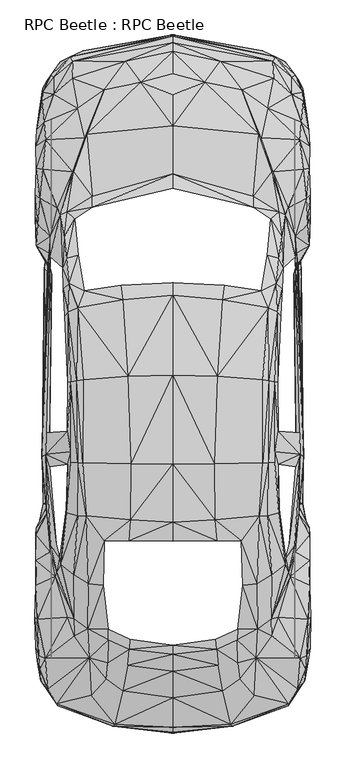
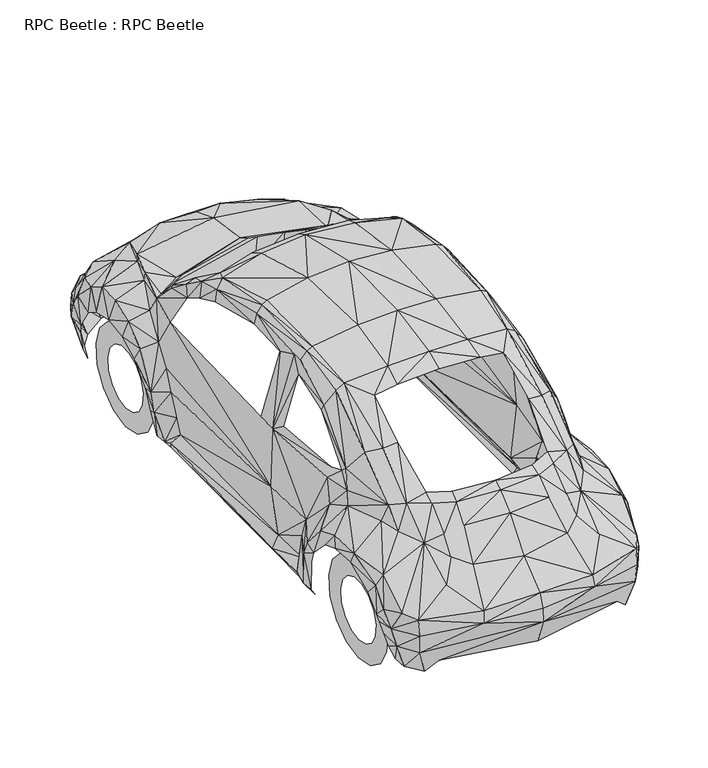
"""IFC4 building model written with IfcOpenShell, lengths in millimetres: proxy geometry, RPC Beetle : RPC Beetle."""

from ifc_helpers import new_model, si_unit, origin, place, context, project, spatial, triangles, source, transform, mapped, element, save


def rpc_beetle_rpc_beetle_31f8b51e(model_context):
    return source(origin(), model_context, "Body", "Tessellation", [
        triangles([(0.0, -748.5640469, 521.3894322), (0.0, -720.14536, 603.624202), (0.0, -696.6746996, 283.1362969), (0.0, -552.698168, 738.4051466), (0.0, -753.249444, 438.4540512), (0.0, -253.6666567, 1039.7136446), (0.0, -401.1024794, 921.3971746), (0.0, -304.8115909, 1012.258271), (0.0, 339.3169338, 1395.7139351), (0.0, 448.6129515, 1442.1297066), (0.0, 778.077507, 1504.0467121), (0.0, 1285.0167675, 1509.4764679), (0.0, 1741.0736687, 1402.3260315), (0.0, 2430.9612099, 967.1999022), (0.0, 3130.000518, 632.0428888), (0.0, 3001.4374352, 771.5092306), (0.0, 2704.2451103, 928.7536297), (0.0, 3164.1993027, 220.1684652), (0.0, 2883.1647125, 858.7358831), (0.0, 3222.5256844, 395.8040746), (0.0, 3178.9998528, 555.7633879), (0.0, 3213.9430687, 530.2784972), (-338.1784132, -715.5037828, 523.0096095), (-331.0409128, -702.1482754, 593.4652654), (-244.7338081, -218.0228295, 1034.0649342), (-248.9812959, -275.9549947, 1002.9312967), (-257.7389917, -368.17353, 911.8513184), (-249.0688632, 342.8199903, 1381.001025), (-285.238149, -511.5370176, 760.4306917), (-240.1360146, 460.0855433, 1426.5848705), (-236.4577871, 780.8799522, 1493.4060825), (-652.4921494, -590.2249108, 370.4943186), (-540.0870918, -593.333878, 283.4428189), (-181.240518, 2954.2772324, 806.3210592), (-253.1849819, 1278.5798058, 1496.1647804), (-379.8650402, -444.3655, 798.2639929), (-370.9321916, -353.3292326, 889.1688366), (-367.9983953, -222.2265337, 1003.4567734), (-368.3924847, -160.7037264, 1036.6922447), (-390.1553641, 342.863774, 1359.0192272), (-282.5670547, 1713.2680984, 1399.3047043), (-397.3366482, 87.4893818, 1215.3492176), (-463.1069432, -537.7663033, 704.8193333), (-271.4885704, 3072.331073, 662.6948696), (-475.7618394, -323.0714138, 849.8468182), (-463.7199872, 3085.9055351, 214.2570346), (-482.2425121, 95.7654028, 1203.3950054), (-485.0449937, -159.3024857, 1005.0769506), (-568.7247697, 3071.499147, 546.7429356), (-493.539933, 483.2496454, 1391.2913853), (-583.2625451, 3099.3922119, 522.0462599), (-510.267146, 3132.2774139, 369.399618), (-391.8631087, 2911.6272194, 782.7628315), (-656.3455479, -597.8441042, 480.0968946), (-660.2426937, -584.8389387, 576.2563957), (-562.2878443, -200.0695649, 879.7105476), (-560.0546594, -101.457906, 987.167506), (-512.4565836, 786.1783207, 1448.435281), (-541.7948364, 484.7822554, 1359.8511532), (-563.9956252, 148.5743069, 1172.305188), (-608.4846974, -561.2369273, 218.4607206), (-511.2742793, 1258.5246346, 1456.1858253), (-542.4078804, 784.6895308, 1430.657151), (-458.8594554, 2304.0621243, 949.0276829), (-601.0406751, -92.7440029, 893.1973698), (-503.7426533, 1765.2887604, 1320.9670441), (-546.0423243, 1253.0073841, 1441.5166626), (-603.011158, 501.1591264, 1278.5798058), (-580.1535416, 788.8932713, 1378.7239838), (-607.2148258, 519.8568223, 1235.1416142), (-601.2595934, 965.2732029, 1337.0374294), (-712.4823103, -503.0858256, 590.4876492), (-542.6706187, 1670.0487888, 1361.1648811), (-490.6061368, 2657.8732315, 893.5038918), (-599.6394161, 778.077507, 1307.3050873), (-598.0630589, 1243.7242298, 1343.7809132), (-639.5745512, 208.1266494, 1062.483621), (-680.4291796, -470.2006963, 218.6796571), (-538.4669146, 1966.7157097, 1180.581209), (-580.9855402, 1248.2344196, 1401.7567348), (-644.5226503, 243.2887836, 1028.2848364), (-502.3414307, 2635.8036484, 866.0047709), (-660.7243504, 162.2363182, 955.24569), (-690.2378105, -396.5922532, 226.8243271), (-559.1350934, 2175.0175301, 1011.1635704), (-670.1826393, 140.8675371, 872.7043619), (-662.475915, 324.2974654, 1009.4558258), (-615.0967575, 1623.4578827, 1262.1154037), (-594.6475333, 1646.0964718, 1321.2735661), (-589.4367322, 1809.6026253, 1269.4280388), (-728.8154703, -481.9797738, 373.2091965), (-751.5854467, -454.4368329, 476.550018), (-694.047389, 315.3208331, 957.7854332), (-726.5822491, -327.3188653, 735.5588814), (-622.9348692, 1777.2429726, 1192.7981958), (-564.6524529, 2445.7178673, 934.1396381), (-731.7930502, -393.8773753, 324.1223308), (-571.0017746, 2444.2728973, 884.1769901), (-698.6452188, 279.8521769, 807.6347145), (-604.2809933, 1949.769651, 1170.4660561), (-587.4224293, 3013.0852707, 200.1133485), (-690.9384218, 574.2421291, 283.6179717), (-750.2280441, -381.0035608, 396.9863425), (-627.532699, 1896.2601265, 1124.7070759), (-602.4856813, 2215.5656364, 949.1590702), (-619.4318127, 2072.8151928, 1075.2699045), (-710.4680437, 549.6329844, 448.6129515), (-764.7219995, -360.335382, 467.5296021), (-699.5209648, 762.6201656, 1015.4986256), (-763.3207769, -313.2189992, 670.9270706), (-757.8472012, -390.9435428, 564.6524529), (-717.4742294, 496.2986309, 583.5690671), (-722.7288506, 461.224064, 180.9777796), (-717.6493641, 554.4497326, 179.883079), (-771.4654106, -341.8128571, 511.011541), (-573.9356071, 2975.4709969, 682.6185808), (-730.7859169, 375.8802907, 185.1814838), (-541.1818288, 2805.3964943, 782.9380388), (-639.7496859, 2198.4444431, 944.2547911), (-738.9305506, 551.5596837, 222.4016865), (-781.5805635, -268.7736925, 609.2290924), (-772.2974092, -106.0556994, 755.9205019), (-721.7217173, 957.7416132, 967.0247675), (-703.3305433, 810.1306377, 292.3318839), (-724.8306845, 835.0462681, 964.3537096), (-757.7596338, 370.5381022, 225.46687), (-785.3463947, -89.9415395, 695.4924316), (-779.6538643, 80.9211054, 675.5686478), (-779.3911623, 89.5036484, 754.6506666), (-760.3869444, 444.1027617, 223.1460814), (-778.077507, 192.1000659, 630.9044409), (-658.6225164, 2237.1534176, 849.7592508), (-770.939934, 345.4910846, 426.1932807), (-774.1802885, 315.1456985, 501.684603), (-781.1864742, 232.2541011, 695.886521), (-719.225794, 810.0868904, 185.8383114), (-689.8874685, 1858.8647346, 293.9082775), (-696.6746996, 1958.8776707, 956.4279579), (-779.7414316, 377.369117, 532.3803311), (-778.1212543, 416.9976937, 439.7239228), (-745.498827, 819.5889267, 613.6517149), (-677.7143017, 2884.8288551, 670.6205486), (-697.5504456, 2077.4130226, 756.8838879), (-639.6182985, 3069.1783585, 391.6879377), (-713.0077869, 1918.2419243, 536.7153863), (-718.1748407, 1909.878336, 192.97583), (-705.1696753, 1981.9541691, 648.2884089), (-730.7859169, 1891.093, 233.3488017), (-673.9922905, 2907.8614609, 198.6683241), (-726.8887711, 2038.9229301, 189.9544301), (-721.6341499, 1973.3715534, 189.9544301), (-678.1959583, 2982.5647499, 540.5250011), (-699.6085321, 2815.6868546, 206.1999501), (-696.3681776, 2991.5851295, 517.4046827), (-723.6484165, 2624.6813622, 787.579616), (-699.0830555, 1882.4667824, 390.3742825), (-764.8971342, 2042.1632847, 362.5686032), (-741.7768158, 2457.6720795, 808.6856678), (-716.1605742, 2965.1367439, 449.5325174), (-766.4297441, 2001.1335217, 376.580902), (-731.5740955, 2724.4316689, 727.6331297), (-771.1588886, 2084.5942703, 482.2425121), (-759.1171091, 2291.4073734, 780.0917736), (-769.0132347, 2143.3146687, 699.0393082), (-777.5520304, 2022.8525448, 494.8098046), (-742.4774271, 2846.864312, 601.8726374), (-782.1060402, 2185.6581596, 616.4542328), (-739.5435946, 2918.4145958, 427.3755486), (-741.1200245, 2896.5202927, 519.8130386), (-750.4031788, 2804.433181, 398.0810795), (-782.2373549, 2313.1701439, 680.7357016), (-778.077507, 2462.7953133, 693.5219124), (-759.9052877, 2786.6113037, 455.2250115), (-774.1802885, 2682.8324638, 602.6608523), (-780.3544756, 2589.4317696, 666.3293135), (-742.6088144, 809.1235044, 220.3874199), (0.0, 2349.0768185, 1011.1635704), (-458.8594554, 2239.9558628, 1006.6095606), (0.0, 1812.0110538, 1368.2148869), (-293.9520611, 1795.8092812, 1359.1506145), (-580.2411452, 849.7154308, 1381.7892036), (338.1784132, -715.5037828, 523.0096095), (331.0409128, -702.1482754, 593.4652654), (244.7338081, -218.0228295, 1034.0649342), (248.9812959, -275.9549947, 1002.9312967), (257.7389917, -368.17353, 911.8513184), (249.0688632, 342.8199903, 1381.001025), (285.238149, -511.5370176, 760.4306917), (240.1360146, 460.0855433, 1426.5848705), (236.4577871, 780.8799522, 1493.4060825), (652.4921494, -590.2249108, 370.4943186), (540.0870918, -593.333878, 283.4428189), (181.240518, 2954.2772324, 806.3210592), (253.1849819, 1278.5798058, 1496.1647804), (379.8650402, -444.3655, 798.2639929), (370.9321916, -353.3292326, 889.1688366), (367.9983953, -222.2265337, 1003.4567734), (368.3924847, -160.7037264, 1036.6922447), (390.1553641, 342.863774, 1359.0192272), (282.5670547, 1713.2680984, 1399.3047043), (397.3366482, 87.4893818, 1215.3492176), (463.1069432, -537.7663033, 704.8193333), (271.4885704, 3072.331073, 662.6948696), (475.7618394, -323.0714138, 849.8468182), (463.7199872, 3085.9055351, 214.2570346), (482.2425121, 95.7654028, 1203.3950054), (485.0449937, -159.3024857, 1005.0769506), (568.7247697, 3071.499147, 546.7429356), (493.539933, 483.2496454, 1391.2913853), (583.2625451, 3099.3922119, 522.0462599), (510.267146, 3132.2774139, 369.399618), (391.8631087, 2911.6272194, 782.7628315), (656.3455479, -597.8441042, 480.0968946), (660.2426937, -584.8389387, 576.2563957), (562.2878443, -200.0695649, 879.7105476), (560.0546594, -101.457906, 987.167506), (512.4565836, 786.1783207, 1448.435281), (541.7948364, 484.7822554, 1359.8511532), (563.9956252, 148.5743069, 1172.305188), (608.4846974, -561.2369273, 218.4607206), (511.2742793, 1258.5246346, 1456.1858253), (542.4078804, 784.6895308, 1430.657151), (458.8594554, 2304.0621243, 949.0276829), (601.0406751, -92.7440029, 893.1973698), (503.7426533, 1765.2887604, 1320.9670441), (546.0423243, 1253.0073841, 1441.5166626), (603.011158, 501.1591264, 1278.5798058), (580.1535416, 788.8932713, 1378.7239838), (607.2148258, 519.8568223, 1235.1416142), (601.2595934, 965.2732029, 1337.0374294), (712.4823103, -503.0858256, 590.4876492), (542.6706187, 1670.0487888, 1361.1648811), (490.6061368, 2657.8732315, 893.5038918), (599.6394161, 778.077507, 1307.3050873), (598.0630589, 1243.7242298, 1343.7809132), (639.5745512, 208.1266494, 1062.483621), (680.4729996, -470.2006963, 218.6796571), (538.4669146, 1966.7157097, 1180.581209), (580.9855402, 1248.2344196, 1401.7567348), (644.5226503, 243.2887836, 1028.2848364), (502.3414307, 2635.8036484, 866.0047709), (660.7243504, 162.2363182, 955.24569), (690.2378105, -396.5922532, 226.8243271), (559.1350934, 2175.0175301, 1011.1635704), (670.1826393, 140.8675371, 872.7043619), (662.475915, 324.2974654, 1009.4558258), (615.0967575, 1623.4578827, 1262.1154037), (594.6475333, 1646.0964718, 1321.2735661), (589.4367322, 1809.6026253, 1269.4280388), (728.8154703, -481.9797738, 373.2091965), (751.5854467, -454.4368329, 476.550018), (694.047389, 315.3208331, 957.7854332), (726.5822491, -327.3188653, 735.5588814), (622.9348692, 1777.2429726, 1192.7981958), (564.6524529, 2445.7178673, 934.1396381), (731.7930502, -393.8773753, 324.1223308), (571.0017746, 2444.2728973, 884.1769901), (698.6452188, 279.8521769, 807.6347145), (604.2809933, 1949.769651, 1170.4660561), (587.4224293, 3013.0852707, 200.1133485), (690.9384218, 574.2421291, 283.6179717), (750.2280441, -381.0035608, 396.9863425), (627.532699, 1896.2601265, 1124.7070759), (602.4856813, 2215.5656364, 949.1590702), (619.4318127, 2072.8151928, 1075.2699045), (710.4680437, 549.6329844, 448.6129515), (764.7219995, -360.335382, 467.5296021), (699.5209648, 762.6201656, 1015.4986256), (763.3207769, -313.2189992, 670.9270706), (757.8472012, -390.9435428, 564.6524529), (717.4742294, 496.2986309, 583.5690671), (722.7288506, 461.224064, 180.9777796), (717.6493641, 554.4497326, 179.883079), (771.4654106, -341.8128571, 511.011541), (573.9356071, 2975.4709969, 682.6185808), (730.7859169, 375.8802907, 185.1814838), (541.1818288, 2805.3964943, 782.9380388), (639.7496859, 2198.4444431, 944.2547911), (738.9305506, 551.5596837, 222.4016865), (781.5805635, -268.7736925, 609.2290924), (772.2974092, -106.0556994, 755.9205019), (721.7654646, 957.7416132, 967.0247675), (703.3305433, 810.1306377, 292.3318839), (724.8306845, 835.0462681, 964.3537096), (757.7596338, 370.5381022, 225.46687), (785.3463947, -89.9415395, 695.4924316), (779.6538643, 80.9211054, 675.5686478), (779.4349096, 89.5036484, 754.6506666), (760.3869444, 444.1027617, 223.1460814), (778.077507, 192.1000659, 630.9044409), (658.6225164, 2237.1534176, 849.7592508), (770.939934, 345.4910846, 426.1932807), (774.1802885, 315.1456985, 501.684603), (781.1864742, 232.2541011, 695.886521), (719.225794, 810.0868904, 185.8383114), (689.8874685, 1858.8647346, 293.9082775), (696.6746996, 1958.8776707, 956.4279579), (779.7414316, 377.369117, 532.3803311), (778.1212543, 416.9976937, 439.7239228), (745.498827, 819.5889267, 613.6517149), (677.7143017, 2884.8288551, 670.6205486), (697.5504456, 2077.4130226, 756.8838879), (639.6182985, 3069.1783585, 391.6879377), (713.0077869, 1918.2419243, 536.7153863), (718.1748407, 1909.878336, 192.97583), (705.1696753, 1981.9541691, 648.2884089), (730.7859169, 1891.093, 233.3488017), (673.9922905, 2907.8614609, 198.6683241), (726.8887711, 2038.9229301, 189.9544301), (721.6341499, 1973.3715534, 189.9544301), (678.1959583, 2982.5647499, 540.5250011), (699.6085321, 2815.6868546, 206.1999501), (696.3681776, 2991.5851295, 517.4046827), (723.6484165, 2624.6813622, 787.579616), (699.0830555, 1882.4667824, 390.3742825), (764.8971342, 2042.1632847, 362.5686032), (741.7768158, 2457.6720795, 808.6856678), (716.1605742, 2965.1367439, 449.5325174), (766.4297441, 2001.1335217, 376.580902), (731.5740955, 2724.4316689, 727.6331297), (771.2027086, 2084.5942703, 482.2425121), (759.1171091, 2291.4073734, 780.0917736), (769.0132347, 2143.3146687, 699.0393082), (777.5520304, 2022.8525448, 494.8098046), (742.4774271, 2846.864312, 601.8726374), (782.1060402, 2185.6581596, 616.4542328), (739.5435946, 2918.4145958, 427.3755486), (741.1200245, 2896.5202927, 519.8130386), (750.4031788, 2804.433181, 398.0810795), (782.2373549, 2313.1701439, 680.7357016), (778.077507, 2462.7953133, 693.5219124), (759.9052877, 2786.6113037, 455.2250115), (774.1802885, 2682.8324638, 602.6608523), (780.3544756, 2589.4317696, 666.3293135), (742.6088144, 809.1235044, 220.3874199), (458.8594554, 2239.9558628, 1006.6095606), (293.9520611, 1795.8092812, 1359.1506145), (580.2411452, 849.7154308, 1381.7892036), (-693.1716431, 2430.2605259, 0.0015107), (-693.1716431, 2430.2605259, 117.8363121), (-693.1716431, 2557.1157188, 26.9752135), (-693.1716431, 2507.7661148, 134.3007777), (-693.1716431, 2661.9892593, 103.1671675), (-693.1716431, 2571.9162689, 180.8917202), (-693.1716431, 2726.8399521, 215.4846123), (-693.1716431, 2611.5449547, 249.552046), (-693.1716431, 2740.4144142, 344.4416937), (-693.1716431, 2619.820903, 328.3713083), (-693.1716431, 2700.3479645, 467.7938301), (-693.1716431, 2595.3430367, 403.7312797), (-693.1716431, 2613.5590759, 564.1285023), (-693.1716431, 2542.3151688, 462.6267763), (-693.1716431, 2495.111364, 616.8935955), (-693.1716431, 2469.8890663, 494.898898), (-693.1716431, 2365.4098331, 616.8935955), (-693.1716431, 2390.6319855, 494.898898), (-693.1716431, 2246.9619759, 564.1285023), (-693.1716431, 2318.205883, 462.6267763), (-693.1716431, 2160.1732327, 467.7938301), (-693.1716431, 2265.1780151, 403.7312797), (-693.1716431, 2120.1067829, 344.4416937), (-693.1716431, 2240.7002941, 328.3713083), (-693.1716431, 2133.681245, 215.4846123), (-693.1716431, 2248.9762424, 249.552046), (-693.1716431, 2198.5319378, 103.1671675), (-693.1716431, 2288.6049282, 180.8917202), (-693.1716431, 2303.4053329, 26.9752135), (-693.1716431, 2352.754937, 134.3007777), (693.1716431, 2430.2605259, 0.0015107), (693.1716431, 2430.2605259, 117.8363121), (693.1716431, 2303.4053329, 26.9752135), (693.1716431, 2352.754937, 134.3007777), (693.1716431, 2198.5319378, 103.1671675), (693.1716431, 2288.6049282, 180.8917202), (693.1716431, 2133.681245, 215.4846123), (693.1716431, 2248.9762424, 249.552046), (693.1716431, 2120.1067829, 344.4416937), (693.1716431, 2240.7002941, 328.3713083), (693.1716431, 2160.1732327, 467.7938301), (693.1716431, 2265.1780151, 403.7312797), (693.1716431, 2246.9619759, 564.1285023), (693.1716431, 2318.205883, 462.6267763), (693.1716431, 2365.4098331, 616.8935955), (693.1716431, 2390.6319855, 494.898898), (693.1716431, 2495.111364, 616.8935955), (693.1716431, 2469.8890663, 494.898898), (693.1716431, 2613.5590759, 564.1285023), (693.1716431, 2542.3151688, 462.6267763), (693.1716431, 2700.3479645, 467.7938301), (693.1716431, 2595.3430367, 403.7312797), (693.1716431, 2740.4144142, 344.4416937), (693.1716431, 2619.820903, 328.3713083), (693.1716431, 2726.8399521, 215.4846123), (693.1716431, 2611.5449547, 249.552046), (693.1716431, 2661.9892593, 103.1671675), (693.1716431, 2571.9162689, 180.8917202), (693.1716431, 2557.1157188, 26.9752135), (693.1716431, 2507.7661148, 134.3007777), (-693.1716431, -13.5744281, 0.0015107), (-693.1716431, -13.5744281, 117.8363121), (-693.1716431, 113.2807944, 26.9752135), (-693.1716431, 63.9311813, 134.3007777), (-693.1716431, 218.1541986, 103.1671675), (-693.1716431, 128.0812991, 180.8917202), (-693.1716431, 283.0049459, 215.4846123), (-693.1716431, 167.7098758, 249.552046), (-693.1716431, 296.5793717, 344.4416937), (-693.1716431, 175.9858968, 328.3713083), (-693.1716431, 256.5129038, 467.7938301), (-693.1716431, 151.5081395, 403.7312797), (-693.1716431, 169.7241424, 564.1285023), (-693.1716431, 98.4802897, 462.6267763), (-693.1716431, 51.2763078, 616.8935955), (-693.1716431, 26.0541442, 494.898898), (-693.1716431, -78.425164, 616.8935955), (-693.1716431, -53.2030025, 494.898898), (-693.1716431, -196.872994, 564.1285023), (-693.1716431, -125.6291504, 462.6267763), (-693.1716431, -283.6617735, 467.7938301), (-693.1716431, -178.6569911, 403.7312797), (-693.1716431, -323.7282414, 344.4416937), (-693.1716431, -203.1347484, 328.3713083), (-693.1716431, -310.1537793, 215.4846123), (-693.1716431, -194.8587274, 249.552046), (-693.1716431, -245.3030684, 103.1671675), (-693.1716431, -155.2301507, 180.8917202), (-693.1716431, -140.4296551, 26.9752135), (-693.1716431, -91.0800329, 134.3007777), (693.1716431, -13.5744281, 0.0015107), (693.1716431, -13.5744281, 117.8363121), (693.1716431, -140.4296551, 26.9752135), (693.1716431, -91.0800329, 134.3007777), (693.1716431, -245.3030684, 103.1671675), (693.1716431, -155.2301507, 180.8917202), (693.1716431, -310.1537793, 215.4846123), (693.1716431, -194.8587274, 249.552046), (693.1716431, -323.7282414, 344.4416937), (693.1716431, -203.1347484, 328.3713083), (693.1716431, -283.6617735, 467.7938301), (693.1716431, -178.6569911, 403.7312797), (693.1716431, -196.872994, 564.1285023), (693.1716431, -125.6291504, 462.6267763), (693.1716431, -78.425164, 616.8935955), (693.1716431, -53.2030025, 494.898898), (693.1716431, 51.2763078, 616.8935955), (693.1716431, 26.0541442, 494.898898), (693.1716431, 169.7241424, 564.1285023), (693.1716431, 98.4802897, 462.6267763), (693.1716431, 256.5129038, 467.7938301), (693.1716431, 151.5081395, 403.7312797), (693.1716431, 296.5793717, 344.4416937), (693.1716431, 175.9858968, 328.3713083), (693.1716431, 283.0049459, 215.4846123), (693.1716431, 167.7098758, 249.552046), (693.1716431, 218.1541986, 103.1671675), (693.1716431, 128.0812991, 180.8917202), (693.1716431, 113.2807944, 26.9752135), (693.1716431, 63.9311813, 134.3007777)], [[67, 58, 62], [67, 63, 58], [53, 82, 74], [34, 17, 19], [118, 82, 53], [155, 98, 82], [155, 158, 98], [34, 74, 17], [172, 155, 175], [172, 158, 155], [159, 168, 169], [166, 142, 169], [175, 161, 174], [175, 155, 161], [142, 152, 169], [154, 169, 152], [160, 145, 165], [160, 156, 145], [162, 160, 165], [162, 157, 160], [34, 53, 74], [74, 96, 64], [82, 96, 74], [82, 98, 96], [36, 29, 27], [29, 43, 24], [23, 55, 54], [23, 24, 55], [23, 2, 24], [23, 1, 2], [5, 1, 23], [134, 140, 133], [134, 139, 140], [117, 130, 113], [117, 126, 130], [113, 120, 114], [113, 130, 120], [140, 112, 107], [140, 139, 112], [92, 108, 103], [91, 103, 97], [91, 92, 103], [61, 33, 32], [84, 78, 91], [84, 91, 97], [38, 26, 25], [77, 81, 83], [63, 50, 58], [63, 59, 50], [68, 63, 69], [68, 59, 63], [181, 75, 69], [74, 64, 17], [64, 14, 17], [64, 178, 14], [178, 177, 14], [34, 19, 16], [53, 34, 44], [21, 44, 15], [21, 49, 44], [44, 34, 15], [34, 16, 15], [22, 49, 21], [22, 51, 49], [20, 51, 22], [20, 52, 51], [18, 52, 20], [18, 46, 52], [51, 152, 49], [51, 154, 152], [101, 144, 46], [144, 52, 46], [101, 159, 144], [159, 169, 154], [101, 168, 159], [101, 149, 168], [149, 170, 168], [149, 153, 170], [168, 173, 169], [168, 170, 173], [49, 142, 116], [49, 152, 142], [49, 116, 44], [116, 142, 118], [161, 155, 118], [155, 82, 118], [142, 161, 118], [158, 132, 98], [158, 163, 132], [172, 163, 158], [172, 171, 163], [98, 119, 96], [98, 132, 119], [171, 164, 163], [171, 167, 164], [163, 143, 132], [163, 164, 143], [96, 105, 64], [96, 119, 105], [105, 178, 64], [105, 85, 178], [167, 165, 164], [167, 162, 165], [165, 143, 164], [165, 147, 143], [150, 160, 157], [150, 151, 160], [151, 156, 160], [151, 148, 137], [13, 35, 12], [13, 41, 35], [12, 31, 11], [12, 35, 31], [35, 58, 31], [35, 62, 58], [11, 30, 10], [11, 31, 30], [31, 50, 30], [31, 58, 50], [10, 28, 9], [10, 30, 28], [30, 40, 28], [30, 50, 40], [125, 75, 181], [125, 109, 75], [125, 87, 109], [125, 93, 87], [123, 141, 125], [137, 141, 156], [137, 124, 141], [148, 124, 137], [148, 176, 124], [146, 176, 148], [146, 136, 176], [141, 112, 125], [112, 93, 125], [112, 99, 93], [124, 112, 141], [124, 107, 112], [124, 102, 107], [176, 102, 124], [176, 120, 102], [136, 120, 176], [136, 114, 120], [47, 40, 50], [47, 42, 40], [48, 42, 47], [48, 39, 42], [57, 47, 60], [57, 48, 47], [60, 50, 59], [60, 47, 50], [59, 77, 60], [59, 68, 77], [77, 57, 60], [77, 83, 57], [70, 77, 68], [70, 81, 77], [75, 68, 69], [75, 70, 68], [26, 6, 25], [26, 8, 6], [27, 8, 26], [27, 7, 8], [29, 7, 27], [29, 4, 7], [24, 4, 29], [24, 2, 4], [32, 5, 23], [33, 5, 32], [33, 3, 5], [32, 23, 54], [55, 45, 72], [55, 24, 43], [99, 83, 93], [99, 86, 83], [135, 86, 99], [135, 129, 86], [131, 129, 135], [131, 128, 129], [93, 81, 87], [93, 83, 81], [128, 122, 129], [128, 127, 122], [122, 86, 129], [122, 65, 86], [86, 57, 83], [86, 65, 57], [127, 110, 122], [127, 121, 110], [110, 94, 122], [122, 94, 65], [94, 56, 65], [56, 57, 65], [56, 48, 57], [56, 45, 48], [94, 45, 56], [115, 110, 121], [115, 111, 110], [111, 94, 110], [111, 72, 94], [108, 92, 115], [92, 111, 115], [78, 32, 91], [78, 61, 32], [45, 38, 48], [45, 37, 38], [37, 26, 38], [37, 27, 26], [36, 27, 37], [134, 135, 139], [134, 131, 135], [139, 99, 112], [139, 135, 99], [126, 140, 130], [126, 133, 140], [130, 107, 120], [130, 140, 107], [120, 107, 102], [45, 36, 37], [92, 55, 72], [92, 54, 55], [91, 54, 92], [91, 32, 54], [92, 72, 111], [72, 45, 94], [43, 45, 55], [43, 36, 45], [43, 29, 36], [79, 90, 66], [79, 100, 90], [90, 73, 66], [85, 100, 79], [85, 106, 100], [85, 105, 106], [105, 119, 106], [95, 88, 89], [90, 89, 73], [89, 67, 73], [73, 67, 62], [89, 76, 80], [89, 80, 67], [88, 76, 89], [73, 35, 41], [73, 62, 35], [69, 63, 181], [80, 63, 67], [76, 71, 80], [146, 148, 151], [141, 147, 145], [151, 137, 156], [173, 166, 169], [173, 174, 166], [166, 174, 161], [166, 161, 142], [52, 144, 51], [144, 154, 51], [144, 159, 154], [116, 53, 44], [116, 118, 53], [119, 143, 138], [143, 119, 132], [143, 147, 138], [138, 104, 119], [119, 104, 106], [104, 100, 106], [104, 90, 100], [104, 95, 90], [95, 89, 90], [25, 39, 38], [38, 39, 48], [141, 138, 147], [156, 141, 145], [165, 145, 147], [41, 179, 180], [41, 13, 179], [66, 41, 180], [66, 73, 41], [123, 125, 71], [125, 181, 71], [71, 181, 80], [181, 63, 80], [138, 141, 123], [226, 221, 217], [226, 217, 222], [212, 233, 241], [193, 19, 17], [277, 212, 241], [314, 241, 257], [314, 257, 317], [193, 17, 233], [331, 334, 314], [331, 314, 317], [318, 328, 327], [325, 328, 301], [334, 333, 320], [334, 320, 314], [301, 328, 311], [313, 311, 328], [319, 324, 304], [319, 304, 315], [321, 324, 319], [321, 319, 316], [193, 233, 212], [233, 223, 255], [241, 233, 255], [241, 255, 257], [195, 186, 188], [188, 183, 202], [182, 213, 214], [182, 214, 183], [182, 183, 2], [182, 2, 1], [5, 182, 1], [293, 292, 299], [293, 299, 298], [276, 272, 289], [276, 289, 285], [272, 273, 279], [272, 279, 289], [299, 266, 271], [299, 271, 298], [251, 262, 267], [250, 256, 262], [250, 262, 251], [220, 191, 192], [243, 250, 237], [243, 256, 250], [197, 184, 185], [236, 242, 240], [222, 217, 209], [222, 209, 218], [227, 228, 222], [227, 222, 218], [338, 228, 234], [233, 17, 223], [223, 17, 14], [223, 14, 336], [336, 14, 177], [193, 16, 19], [212, 203, 193], [21, 15, 203], [21, 203, 208], [203, 15, 193], [193, 15, 16], [22, 21, 208], [22, 208, 210], [20, 22, 210], [20, 210, 211], [18, 20, 211], [18, 211, 205], [210, 208, 311], [210, 311, 313], [260, 205, 303], [303, 205, 211], [260, 303, 318], [318, 313, 328], [260, 318, 327], [260, 327, 308], [308, 327, 329], [308, 329, 312], [327, 328, 332], [327, 332, 329], [208, 275, 301], [208, 301, 311], [208, 203, 275], [275, 277, 301], [320, 277, 314], [314, 277, 241], [301, 277, 320], [317, 257, 291], [317, 291, 322], [331, 317, 322], [331, 322, 330], [257, 255, 278], [257, 278, 291], [330, 322, 323], [330, 323, 326], [322, 291, 302], [322, 302, 323], [255, 223, 264], [255, 264, 278], [264, 223, 336], [264, 336, 244], [326, 323, 324], [326, 324, 321], [324, 323, 302], [324, 302, 306], [309, 316, 319], [309, 319, 310], [310, 319, 315], [310, 296, 307], [13, 12, 194], [13, 194, 200], [12, 11, 190], [12, 190, 194], [194, 190, 217], [194, 217, 221], [11, 10, 189], [11, 189, 190], [190, 189, 209], [190, 209, 217], [10, 9, 187], [10, 187, 189], [189, 187, 199], [189, 199, 209], [284, 338, 234], [284, 234, 268], [284, 268, 246], [284, 246, 252], [282, 284, 300], [296, 315, 300], [296, 300, 283], [307, 296, 283], [307, 283, 335], [305, 307, 335], [305, 335, 295], [300, 284, 271], [271, 284, 252], [271, 252, 258], [283, 300, 271], [283, 271, 266], [283, 266, 261], [335, 283, 261], [335, 261, 279], [295, 335, 279], [295, 279, 273], [206, 209, 199], [206, 199, 201], [207, 206, 201], [207, 201, 198], [216, 219, 206], [216, 206, 207], [219, 218, 209], [219, 209, 206], [218, 219, 236], [218, 236, 227], [236, 219, 216], [236, 216, 242], [229, 227, 236], [229, 236, 240], [234, 228, 227], [234, 227, 229], [185, 184, 6], [185, 6, 8], [186, 185, 8], [186, 8, 7], [188, 186, 7], [188, 7, 4], [183, 188, 4], [183, 4, 2], [191, 182, 5], [192, 191, 5], [192, 5, 3], [191, 213, 182], [214, 231, 204], [214, 202, 183], [258, 252, 242], [258, 242, 245], [294, 258, 245], [294, 245, 288], [290, 294, 288], [290, 288, 287], [252, 246, 240], [252, 240, 242], [287, 288, 281], [287, 281, 286], [281, 288, 245], [281, 245, 224], [245, 242, 216], [245, 216, 224], [286, 281, 269], [286, 269, 280], [269, 281, 253], [281, 224, 253], [253, 224, 215], [215, 224, 216], [215, 216, 207], [215, 207, 204], [253, 215, 204], [274, 280, 269], [274, 269, 270], [270, 269, 253], [270, 253, 231], [267, 274, 251], [251, 274, 270], [237, 250, 191], [237, 191, 220], [204, 207, 197], [204, 197, 196], [196, 197, 185], [196, 185, 186], [195, 196, 186], [293, 298, 294], [293, 294, 290], [298, 271, 258], [298, 258, 294], [285, 289, 299], [285, 299, 292], [289, 279, 266], [289, 266, 299], [279, 261, 266], [204, 196, 195], [251, 231, 214], [251, 214, 213], [250, 251, 213], [250, 213, 191], [251, 270, 231], [231, 253, 204], [202, 214, 204], [202, 204, 195], [202, 195, 188], [238, 225, 249], [238, 249, 259], [249, 225, 232], [244, 238, 259], [244, 259, 265], [244, 265, 264], [264, 265, 278], [254, 248, 247], [249, 232, 248], [248, 232, 226], [232, 221, 226], [248, 239, 235], [248, 226, 239], [247, 248, 235], [232, 200, 194], [232, 194, 221], [228, 338, 222], [239, 226, 222], [235, 239, 230], [305, 310, 307], [300, 304, 306], [310, 315, 296], [332, 328, 325], [332, 325, 333], [325, 320, 333], [325, 301, 320], [211, 210, 303], [303, 210, 313], [303, 313, 318], [275, 203, 212], [275, 212, 277], [278, 297, 302], [302, 291, 278], [302, 297, 306], [297, 278, 263], [278, 265, 263], [263, 265, 259], [263, 259, 249], [263, 249, 254], [254, 249, 248], [184, 197, 198], [197, 207, 198], [300, 306, 297], [315, 304, 300], [324, 306, 304], [200, 337, 179], [200, 179, 13], [225, 337, 200], [225, 200, 232], [282, 230, 284], [284, 230, 338], [230, 239, 338], [338, 239, 222], [297, 282, 300], [339, 342, 341], [339, 340, 342], [341, 344, 343], [341, 342, 344], [343, 346, 345], [343, 344, 346], [345, 348, 347], [345, 346, 348], [347, 350, 349], [347, 348, 350], [349, 352, 351], [349, 350, 352], [351, 354, 353], [351, 352, 354], [353, 356, 355], [353, 354, 356], [355, 358, 357], [355, 356, 358], [357, 360, 359], [357, 358, 360], [359, 362, 361], [359, 360, 362], [361, 364, 363], [361, 362, 364], [363, 366, 365], [363, 364, 366], [365, 368, 367], [365, 366, 368], [367, 340, 339], [367, 368, 340], [369, 372, 371], [369, 370, 372], [371, 374, 373], [371, 372, 374], [373, 376, 375], [373, 374, 376], [375, 378, 377], [375, 376, 378], [377, 380, 379], [377, 378, 380], [379, 382, 381], [379, 380, 382], [381, 384, 383], [381, 382, 384], [383, 386, 385], [383, 384, 386], [385, 388, 387], [385, 386, 388], [387, 390, 389], [387, 388, 390], [389, 392, 391], [389, 390, 392], [391, 394, 393], [391, 392, 394], [393, 396, 395], [393, 394, 396], [395, 398, 397], [395, 396, 398], [397, 370, 369], [397, 398, 370], [399, 402, 401], [399, 400, 402], [401, 404, 403], [401, 402, 404], [403, 406, 405], [403, 404, 406], [405, 408, 407], [405, 406, 408], [407, 410, 409], [407, 408, 410], [409, 412, 411], [409, 410, 412], [411, 414, 413], [411, 412, 414], [413, 416, 415], [413, 414, 416], [415, 418, 417], [415, 416, 418], [417, 420, 419], [417, 418, 420], [419, 422, 421], [419, 420, 422], [421, 424, 423], [421, 422, 424], [423, 426, 425], [423, 424, 426], [425, 428, 427], [425, 426, 428], [427, 400, 399], [427, 428, 400], [429, 432, 431], [429, 430, 432], [431, 434, 433], [431, 432, 434], [433, 436, 435], [433, 434, 436], [435, 438, 437], [435, 436, 438], [437, 440, 439], [437, 438, 440], [439, 442, 441], [439, 440, 442], [441, 444, 443], [441, 442, 444], [443, 446, 445], [443, 444, 446], [445, 448, 447], [445, 446, 448], [447, 450, 449], [447, 448, 450], [449, 452, 451], [449, 450, 452], [451, 454, 453], [451, 452, 454], [453, 456, 455], [453, 454, 456], [455, 458, 457], [455, 456, 458], [457, 430, 429], [457, 458, 430]], closed=False),
    ])


if __name__ == "__main__":
    model = new_model("IFC4")
    model_context = context("Model", 3, world=origin())
    ifc_project = project(units=[si_unit("LENGTHUNIT", "METRE", prefix="MILLI")], contexts=[model_context])
    site = spatial("IfcSite", under=ifc_project)
    building = spatial("IfcBuilding", under=site)
    placement = place(None, origin())
    rpc_beetle_rpc_beetle_shape = rpc_beetle_rpc_beetle_31f8b51e(model_context)
    element("IfcBuildingElementProxy", 1, Name="RPC Beetle : RPC Beetle", ObjectType="RPC Beetle : RPC Beetle", at=placement, inside=building, context=model_context, shape_type="MappedRepresentation", body=[
        mapped(rpc_beetle_rpc_beetle_shape, transform((0.0, 0.0, 0.0), x_axis=(1.0, 0.0, 0.0), y_axis=(0.0, 1.0, 0.0), z_axis=(0.0, 0.0, 1.0))),
    ])
    save(model, "model.ifc")

# Revit data of these elements
# Type "RPC Beetle : RPC Beetle"
#   built-in parameter 1005198 = "{2, 15},{39, RPC-16-0U6E-L4EG-ENH1-J3KF-SVEL-0TX4-C0},{1, 0},{1, 0},{2, 34},{2, 11},{20, AdvancedUIDefinition},{1, 0},{1, 0},{0, },{2, 11},{10, AssetLibID},{1, 0},{1, 0},{36, 4D3F6E72-3F99-4203-98E9-AF80B3C7A7A4},{2, 11},{10, BaseSchema},{1, 0},{1, 0},{9, RPCSchema},{2, 11},{12, ExchangeGUID},{1, 0},{1, 0},{0, },{1, 2},{6, Hidden},{1, 0},{1, 0},{1, 0},{2, 11},{12, LocalizedUID},{1, 0},{1, 0},{0, },{1, 4},{11, RPCCategory},{1, 0},{1, 0},{1, 0},{2, 11},{11, RPCFilePath},{1, 0},{1, 0},{115, C:\\Program Files\\Common Files\\Autodesk Shared\\Materials\\4\\assetlibrary_base.fbm\\RPCs\\ArchVision_Demo_VW_Beetle4.rpc},{2, 11},{8, RPCImage},{1, 0},{1, 0},{0, },{1, 6},{14, RPCPlantHeight},{1, 0},{1, 0},{1, 0},{2, 11},{9, RPCTypeId},{1, 0},{1, 0},{39, RPC-16-0U6E-L4EG-ENH1-J3KF-SVEL-0TX4-C0},{1, 4},{13, SchemaVersion},{1, 0},{1, 0},{1, 5},{2, 11},{12, UIDefinition},{1, 0},{1, 0},{0, },{2, 11},{6, UIName},{1, 0},{1, 0},{39, RPC-16-0U6E-L4EG-ENH1-J3KF-SVEL-0TX4-C0},{2, 11},{11, VersionGUID},{1, 0},{1, 0},{9, RPCSchema},{2, 11},{9, assettype},{1, 0},{1, 0},{11, RPCGeometry},{2, 11},{8, category},{1, 0},{1, 0},{21, :Auto_Economy/Midsize},{2, 11},{11, description},{1, 0},{1, 0},{0, },{2, 11},{7, keyword},{1, 0},{1, 0},{27, :Geometry:RPC:VW Beetle [4]},{2, 11},{9, localname},{1, 0},{1, 0},{3, RPC},{2, 11},{9, localtype},{1, 0},{1, 0},{3, RPC},{1, 4},{8, revision},{1, 0},{1, 0},{1, 1},{2, 11},{9, thumbnail},{1, 0},{1, 0},{0, },{1, 4},{7, version},{1, 0},{1, 0},{1, 1},{2, 14},{6, Height},{1, 0},{1, 0},{7, 4.91667},{1, 2},{20, RPC_Cast Reflections},{1, 0},{1, 0},{1, 1},{1, 4},{16, RPC_Transparency},{1, 0},{1, 0},{2, 14},{1, 4},{11, RPC_Tinting},{1, 0},{1, 0},{2, 44},{1, 2},{15, RPC_Use Tinting},{1, 0},{1, 0},{1, 0},{1, 2},{17, RPC_License Plate},{1, 0},{1, 0},{1, 0},{2, 11},{25, RPC_License Plate Texture},{1, 0},{1, 0},{64, __RPC:/object data/textures/car/plate/textures/default/rgb/0/0/0},{2, 11},{27, RPC_i_License Plate Texture},{1, 0},{1, 0},{0, },{1, 2},{16, RPC_Custom Plate},{1, 0},{1, 0},{1, 0},{2, 11},{27, RPC_License Plate File Name},{1, 0},{1, 0},{0, },{21, assetlibrary_base.fbx},{1, 5},"
#   built-in parameter 1005195 = "RPC-16-0U6E-L4EG-ENH1-J3KF-SVEL-0TX4-C0"
#   Height = 0
